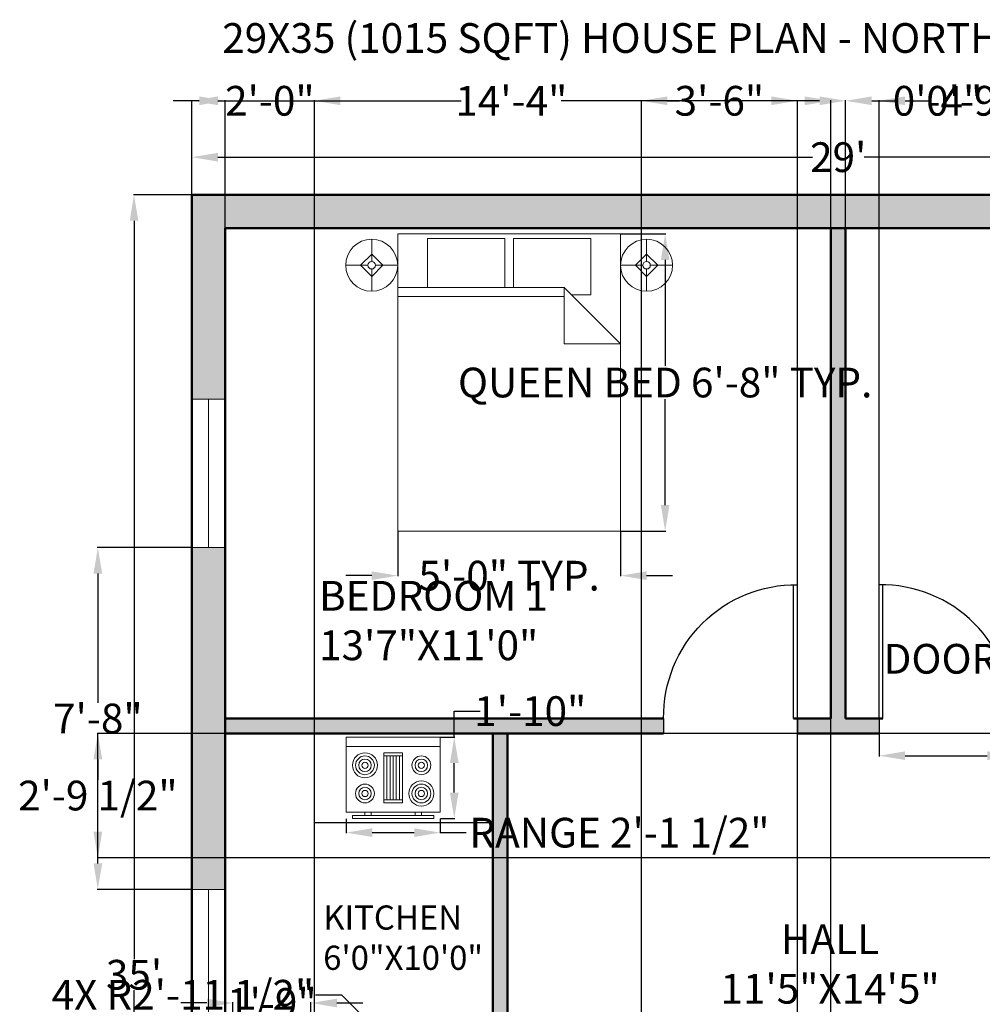
# Model space of a CAD drawing. Units: inches. Extents: x 808573 to 809030, y 884276 to 884799.
# Tile 3 of 4: x 808573 to 808832, y 884534 to 884799. Entities that reach past the tile are written whole.
import ezdxf

# ---------------------------------------------------------------- set-up
doc = ezdxf.new("R2010")
doc.units = ezdxf.units.IN
doc.header["$MEASUREMENT"] = 0
for name, color, linetype, lineweight in [('A-ANNO-DIMS', 2, 'Continuous', 18), ('A-ANNO-TEXT', 7, 'Continuous', 25), ('A-AREA-IDEN', 7, 'Continuous', 25), ('A-DOOR', 3, 'Continuous', 25), ('A-EQPM', 9, 'Continuous', 18), ('A-FLOR-CASE', 9, 'Continuous', 25), ('A-FURN', 8, 'Continuous', 18), ('A-GLAZ', 4, 'Continuous', 18), ('A-WALL', 7, 'Continuous', 50)]:
    doc.layers.add(name, color=color, linetype=linetype, lineweight=lineweight)
doc.layers.add('A-WALL-PATT', color=251, linetype='Continuous', lineweight=13, true_color=0x636466)
doc.styles.get("Standard").update_dxf_attribs({"font": 'arial.ttf'})
doc.dimstyles.get("Standard").update_dxf_attribs({"dimtxt": 8, "dimasz": 7, "dimexe": 0.18, "dimexo": 0.0625, "dimgap": 0.09, "dimtad": 0, "dimtih": 1, "dimtoh": 1, "dimdec": 0, "dimzin": 0, "dimdsep": 46, "dimlunit": 3, "dimtxsty": 'Standard', "dimcen": 0.09, "dimadec": 0, "dimazin": 0, "dimtfac": 1, "dimtdec": 0, "dimtofl": 0, "dimtmove": 0, "dimatfit": 3, "dimfxl": 1, "dimtolj": 1, "dimtzin": 0, "dimarcsym": 0})

# ---------------------------------------------------------------- blocks, each defined once
blk = doc.blocks.new('Range-Oven - 30 in top')
for p, q in [((0, -3), (30, -3)), ((12, -6), (18, -6)), ((13, -20), (13, -6)), ((14, -6), (14, -20)), ((15, -20), (15, -6)), ((16, -6), (16, -20)), ((17, -20), (17, -6)), ((18, -20), (12, -20)), ((6, -24), (6, -25)), ((8, -25), (8, -24)), ((22, -25), (22, -24)), ((24, -24), (24, -25))]:
    blk.add_line(p, q)
for points in [[(0, -24), (0, 0), (30, 0), (30, -24)], [(12, -21), (12, -5), (18, -5), (18, -21)], [(2, -26), (2, -25), (28, -25), (28, -26)]]:
    blk.add_lwpolyline(points, close=True)
for centre, radius in [((6, -9), 4), ((6, -9), 3), ((24, -9), 3), ((6, -9), 2), ((6, -9), 1), ((24, -9), 2), ((24, -9), 1), ((6, -18), 3), ((24, -18), 4), ((24, -18), 3), ((6, -18), 2), ((6, -18), 1), ((24, -18), 2), ((24, -18), 1)]:
    blk.add_circle(centre, radius)
blk = doc.blocks.new('Bed - Queen')
for p, q in [((0, -80.00003), (0, 0)), ((0, 0), (59.99999, 0)), ((59.99999, 0), (59.99999, -80.00003)), ((7.99999, -1.2), (28.79998, -1.2)), ((7.99999, -14.4), (7.99999, -1.2)), ((28.79998, -1.2), (28.79998, -14.4)), ((31.19999, -1.2), (51.99999, -1.2)), ((31.19999, -14.4), (31.19999, -1.2)), ((51.99999, -1.2), (51.99999, -16.4)), ((0, -14.4), (44.8, -14.4)), ((59.99999, -29.6), (44.8, -14.4)), ((44.8, -14.4), (44.8, -29.6)), ((44.8, -16.8), (0, -16.8)), ((51.99999, -16.4), (46.79936, -16.4)), ((44.8, -29.6), (59.99999, -29.6)), ((59.99999, -80.00003), (0, -80.00003))]:
    blk.add_line(p, q)
blk = doc.blocks.new('Lamp - Table')
for p, q in [((0, 7), (0, 1)), ((0, 3), (-3, 0)), ((3, 0), (0, 3)), ((-1, 0), (-7, 0)), ((-3, 0), (0, -3)), ((0, -3), (3, 0)), ((1, 0), (7, 0)), ((0, -1), (0, -7))]:
    blk.add_line(p, q)
for radius in [7, 1]:
    blk.add_circle((0, 0), radius)
blk = doc.blocks.new('*D6')
at = {"layer": 'A-ANNO-DIMS', "color": 0, "lineweight": -2, "transparency": 16777216}
for p, q in [((808619.63, 884751.7), (808619.63, 884761.94)), ((808626.63, 884761.76), (808786.68, 884761.76)), ((808960.63, 884761.76), (808800.58, 884761.76)), ((808967.63, 884751.7), (808967.63, 884761.94))]:
    blk.add_line(p, q, dxfattribs=at)
at = {"layer": 'A-ANNO-DIMS', "color": 0, "transparency": 16777216}
for points in [[(808626.63, 884762.92), (808626.63, 884760.59), (808619.63, 884761.76)], [(808960.63, 884762.92), (808960.63, 884760.59), (808967.63, 884761.76)]]:
    blk.add_solid(points, dxfattribs=at)
at = {"layer": 'Defpoints', "color": 0, "transparency": 16777216}
for p in [(808967.63, 884761.76), (808619.63, 884751.64), (808967.63, 884751.64)]:
    blk.add_point(p, dxfattribs=at)
at = {"layer": 'A-ANNO-DIMS', "color": 0, "transparency": 16777216, "insert": (808793.63, 884761.76), "char_height": 8, "attachment_point": 5}
blk.add_mtext("\\A1;29'", dxfattribs=at)
blk = doc.blocks.new('*D7')
at = {"layer": 'A-ANNO-DIMS', "color": 0, "lineweight": -2, "transparency": 16777216}
for p, q in [((808619.57, 884751.64), (808603.89, 884751.64)), ((808604.07, 884744.64), (808604.07, 884545.82)), ((808604.07, 884338.64), (808604.07, 884537.46)), ((808619.57, 884331.64), (808603.89, 884331.64))]:
    blk.add_line(p, q, dxfattribs=at)
at = {"layer": 'A-ANNO-DIMS', "color": 0, "transparency": 16777216}
for points in [[(808602.9, 884744.64), (808605.23, 884744.64), (808604.07, 884751.64)], [(808602.9, 884338.64), (808605.23, 884338.64), (808604.07, 884331.64)]]:
    blk.add_solid(points, dxfattribs=at)
at = {"layer": 'Defpoints', "color": 0, "transparency": 16777216}
for p in [(808619.63, 884751.64), (808604.07, 884331.64), (808619.63, 884331.64)]:
    blk.add_point(p, dxfattribs=at)
at = {"layer": 'A-ANNO-DIMS', "color": 0, "transparency": 16777216, "insert": (808604.07, 884541.64), "char_height": 8, "attachment_point": 5}
blk.add_mtext("\\A1;35'", dxfattribs=at)
blk = doc.blocks.new('DOOR-SWING-36IN')
for p, q in [((0, 0), (0, 36)), ((1, 0), (1, 36)), ((0, 0), (0, -4)), ((36, 0), (36, -4))]:
    blk.add_line(p, q)
blk.add_arc((0.5, 0.5), 35.5, 359.1931, 90.8069)
blk = doc.blocks.new('WIN-40IN')
for p, q in [((0, 0), (9, 0)), ((4.5, 0), (4.5, -40)), ((0, -40), (9, -40))]:
    blk.add_line(p, q)
blk = doc.blocks.new('WIN-36IN')
for p, q in [((0, 0), (-9, 0)), ((-4.5, 0), (-4.5, -36)), ((0, -36), (-9, -36))]:
    blk.add_line(p, q)
blk = doc.blocks.new('*D17')
at = {"layer": 'A-ANNO-DIMS', "color": 0, "lineweight": -2, "transparency": 16777216}
for p, q in [((808735.1, 884741.09), (808747.22, 884741.09)), ((808747.04, 884734.09), (808747.04, 884705.56)), ((808747.04, 884668.09), (808747.04, 884696.62)), ((808735.1, 884661.09), (808747.22, 884661.09))]:
    blk.add_line(p, q, dxfattribs=at)
at = {"layer": 'A-ANNO-DIMS', "color": 0, "transparency": 16777216}
for points in [[(808745.88, 884734.09), (808748.21, 884734.09), (808747.04, 884741.09)], [(808745.88, 884668.09), (808748.21, 884668.09), (808747.04, 884661.09)]]:
    blk.add_solid(points, dxfattribs=at)
at = {"layer": 'Defpoints', "color": 0, "transparency": 16777216}
for p in [(808735.04, 884741.09), (808747.04, 884741.09), (808735.04, 884661.09)]:
    blk.add_point(p, dxfattribs=at)
at = {"layer": 'A-ANNO-DIMS', "color": 0, "transparency": 16777216, "insert": (808747.04, 884701.09), "char_height": 8, "attachment_point": 5}
blk.add_mtext('\\A1;QUEEN BED 6\'-8" TYP.', dxfattribs=at)
blk = doc.blocks.new('*D18')
at = {"layer": 'A-ANNO-DIMS', "color": 0, "lineweight": -2, "transparency": 16777216}
for p, q in [((808675.04, 884661.03), (808675.04, 884648.91)), ((808735.04, 884661.03), (808735.04, 884648.91)), ((808668.04, 884649.09), (808661.04, 884649.09)), ((808742.04, 884649.09), (808749.04, 884649.09))]:
    blk.add_line(p, q, dxfattribs=at)
at = {"layer": 'A-ANNO-DIMS', "color": 0, "transparency": 16777216}
for points in [[(808668.04, 884650.26), (808668.04, 884647.92), (808675.04, 884649.09)], [(808742.04, 884650.26), (808742.04, 884647.92), (808735.04, 884649.09)]]:
    blk.add_solid(points, dxfattribs=at)
at = {"layer": 'Defpoints', "color": 0, "transparency": 16777216}
for p in [(808675.04, 884661.09), (808735.04, 884661.09), (808735.04, 884649.09)]:
    blk.add_point(p, dxfattribs=at)
at = {"layer": 'A-ANNO-DIMS', "color": 0, "transparency": 16777216, "insert": (808705.04, 884649.09), "char_height": 8, "attachment_point": 5}
blk.add_mtext('\\A1;5\'-0" TYP.', dxfattribs=at)
blk = doc.blocks.new('*D19')
at = {"layer": 'A-ANNO-DIMS', "color": 0, "lineweight": -2, "transparency": 16777216}
for p, q in [((808840.83, 884646.78), (808846.96, 884646.78)), ((808846.78, 884639.78), (808846.78, 884630.94)), ((808846.78, 884613.64), (808846.78, 884622.48)), ((808840.83, 884606.64), (808846.96, 884606.64))]:
    blk.add_line(p, q, dxfattribs=at)
at = {"layer": 'A-ANNO-DIMS', "color": 0, "transparency": 16777216}
for points in [[(808845.62, 884639.78), (808847.95, 884639.78), (808846.78, 884646.78)], [(808845.62, 884613.64), (808847.95, 884613.64), (808846.78, 884606.64)]]:
    blk.add_solid(points, dxfattribs=at)
at = {"layer": 'Defpoints', "color": 0, "transparency": 16777216}
for p in [(808840.76, 884646.78), (808846.78, 884646.78), (808840.76, 884606.64)]:
    blk.add_point(p, dxfattribs=at)
at = {"layer": 'A-ANNO-DIMS', "color": 0, "transparency": 16777216, "insert": (808846.78, 884626.71), "char_height": 8, "attachment_point": 5}
blk.add_mtext('\\A1;DOOR 3\'-4" TYP.', dxfattribs=at)
blk = doc.blocks.new('*D20')
at = {"layer": 'A-ANNO-DIMS', "color": 0, "lineweight": -2, "transparency": 16777216}
for p, q in [((808804.63, 884606.58), (808804.63, 884600.44)), ((808840.76, 884606.58), (808840.76, 884600.44)), ((808811.63, 884600.62), (808833.76, 884600.62)), ((808840.76, 884600.62), (808847.76, 884600.62))]:
    blk.add_line(p, q, dxfattribs=at)
at = {"layer": 'A-ANNO-DIMS', "color": 0, "transparency": 16777216}
for points in [[(808811.63, 884601.79), (808811.63, 884599.45), (808804.63, 884600.62)], [(808833.76, 884601.79), (808833.76, 884599.45), (808840.76, 884600.62)]]:
    blk.add_solid(points, dxfattribs=at)
at = {"layer": 'Defpoints', "color": 0, "transparency": 16777216}
for p in [(808804.63, 884606.64), (808840.76, 884606.64), (808840.76, 884600.62)]:
    blk.add_point(p, dxfattribs=at)
at = {"layer": 'A-ANNO-DIMS', "color": 0, "transparency": 16777216, "insert": (808872.23, 884600.62), "char_height": 8, "attachment_point": 5}
blk.add_mtext('\\A1;3\'-0" TYP.', dxfattribs=at)
blk = doc.blocks.new('*D29')
at = {"layer": 'A-ANNO-DIMS', "color": 0, "lineweight": -2, "transparency": 16777216}
for p, q in [((808661.18, 884583.63), (808661.18, 884579.72)), ((808686.48, 884583.63), (808686.48, 884579.72)), ((808668.18, 884579.9), (808679.48, 884579.9)), ((808686.48, 884579.9), (808693.48, 884579.9))]:
    blk.add_line(p, q, dxfattribs=at)
at = {"layer": 'A-ANNO-DIMS', "color": 0, "transparency": 16777216}
for points in [[(808668.18, 884581.07), (808668.18, 884578.74), (808661.18, 884579.9)], [(808679.48, 884581.07), (808679.48, 884578.74), (808686.48, 884579.9)]]:
    blk.add_solid(points, dxfattribs=at)
at = {"layer": 'Defpoints', "color": 0, "transparency": 16777216}
for p in [(808661.18, 884583.7), (808686.48, 884583.7), (808686.48, 884579.9)]:
    blk.add_point(p, dxfattribs=at)
at = {"layer": 'A-ANNO-DIMS', "color": 0, "transparency": 16777216, "insert": (808734.74, 884579.9), "char_height": 8, "attachment_point": 5}
blk.add_mtext('\\A1;RANGE 2\'-1 1/2"', dxfattribs=at)
blk = doc.blocks.new('*D30')
at = {"layer": 'A-ANNO-DIMS', "color": 0, "lineweight": -2, "transparency": 16777216}
for p, q in [((808690.27, 884605.62), (808690.27, 884612.62)), ((808690.27, 884612.62), (808697.27, 884612.62)), ((808686.54, 884605.62), (808690.45, 884605.62)), ((808690.27, 884590.7), (808690.27, 884598.62)), ((808686.54, 884583.7), (808690.45, 884583.7))]:
    blk.add_line(p, q, dxfattribs=at)
at = {"layer": 'A-ANNO-DIMS', "color": 0, "transparency": 16777216}
for points in [[(808689.1, 884598.62), (808691.44, 884598.62), (808690.27, 884605.62)], [(808689.1, 884590.7), (808691.44, 884590.7), (808690.27, 884583.7)]]:
    blk.add_solid(points, dxfattribs=at)
at = {"layer": 'Defpoints', "color": 0, "transparency": 16777216}
for p in [(808686.48, 884605.62), (808690.27, 884605.62), (808686.48, 884583.7)]:
    blk.add_point(p, dxfattribs=at)
at = {"layer": 'A-ANNO-DIMS', "color": 0, "transparency": 16777216, "insert": (808710.73, 884612.62), "char_height": 8, "attachment_point": 5}
blk.add_mtext('\\A1;1\'-10"', dxfattribs=at)
blk = doc.blocks.new('*D32')
at = {"layer": 'A-ANNO-DIMS', "color": 0, "lineweight": -2, "transparency": 16777216}
for p, q in [((808623.67, 884534.04), (808616.67, 884534.04)), ((808630.67, 884528.7), (808630.67, 884534.22)), ((808651.67, 884528.7), (808651.67, 884534.22)), ((808658.67, 884534.04), (808665.67, 884534.04))]:
    blk.add_line(p, q, dxfattribs=at)
at = {"layer": 'A-ANNO-DIMS', "color": 0, "transparency": 16777216}
for points in [[(808623.67, 884535.2), (808623.67, 884532.87), (808630.67, 884534.04)], [(808658.67, 884535.2), (808658.67, 884532.87), (808651.67, 884534.04)]]:
    blk.add_solid(points, dxfattribs=at)
at = {"layer": 'Defpoints', "color": 0, "transparency": 16777216}
for p in [(808651.67, 884534.04), (808630.67, 884528.64), (808651.67, 884528.64)]:
    blk.add_point(p, dxfattribs=at)
at = {"layer": 'A-ANNO-DIMS', "color": 0, "transparency": 16777216, "insert": (808641.17, 884534.04), "char_height": 8, "attachment_point": 5}
blk.add_mtext('\\A1;1\'-9"', dxfattribs=at)
blk = doc.blocks.new('*D35')
at = {"layer": 'A-ANNO-DIMS', "color": 0, "lineweight": -2, "transparency": 16777216}
for p, q in [((808619.57, 884656.64), (808594.15, 884656.64)), ((808594.33, 884649.64), (808594.33, 884614.81)), ((808594.33, 884571.64), (808594.33, 884606.47)), ((808619.57, 884564.64), (808594.15, 884564.64))]:
    blk.add_line(p, q, dxfattribs=at)
at = {"layer": 'A-ANNO-DIMS', "color": 0, "transparency": 16777216}
for points in [[(808593.16, 884649.64), (808595.5, 884649.64), (808594.33, 884656.64)], [(808593.16, 884571.64), (808595.5, 884571.64), (808594.33, 884564.64)]]:
    blk.add_solid(points, dxfattribs=at)
at = {"layer": 'Defpoints', "color": 0, "transparency": 16777216}
for p in [(808594.33, 884656.64), (808619.63, 884656.64), (808619.63, 884564.64)]:
    blk.add_point(p, dxfattribs=at)
at = {"layer": 'A-ANNO-DIMS', "color": 0, "transparency": 16777216, "insert": (808594.33, 884610.64), "char_height": 8, "attachment_point": 5}
blk.add_mtext('\\A1;7\'-8"', dxfattribs=at)
blk = doc.blocks.new('*D40')
at = {"layer": 'A-ANNO-DIMS', "color": 0, "lineweight": -2, "transparency": 16777216}
for p, q in [((808619.63, 884331.7), (808619.63, 884777.12)), ((808626.63, 884776.94), (808692.17, 884776.94)), ((808784.63, 884776.94), (808719.08, 884776.94)), ((808791.63, 884331.7), (808791.63, 884777.12))]:
    blk.add_line(p, q, dxfattribs=at)
at = {"layer": 'A-ANNO-DIMS', "color": 0, "transparency": 16777216}
for points in [[(808626.63, 884778.11), (808626.63, 884775.77), (808619.63, 884776.94)], [(808784.63, 884778.11), (808784.63, 884775.77), (808791.63, 884776.94)]]:
    blk.add_solid(points, dxfattribs=at)
at = {"layer": 'Defpoints', "color": 0, "transparency": 16777216}
for p in [(808791.63, 884776.94), (808619.63, 884331.64), (808791.63, 884331.64)]:
    blk.add_point(p, dxfattribs=at)
at = {"layer": 'A-ANNO-DIMS', "color": 0, "transparency": 16777216, "insert": (808705.63, 884776.94), "char_height": 8, "attachment_point": 5}
blk.add_mtext('\\A1;14\'-4"', dxfattribs=at)
blk = doc.blocks.new('*D45')
at = {"layer": 'A-ANNO-DIMS', "color": 0, "lineweight": -2, "transparency": 16777216}
for p, q in [((808784.63, 884776.94), (808777.63, 884776.94)), ((808791.63, 884742.7), (808791.63, 884777.12)), ((808795.63, 884742.7), (808795.63, 884777.12)), ((808802.63, 884776.94), (808809.63, 884776.94))]:
    blk.add_line(p, q, dxfattribs=at)
at = {"layer": 'A-ANNO-DIMS', "color": 0, "transparency": 16777216}
for points in [[(808784.63, 884778.11), (808784.63, 884775.77), (808791.63, 884776.94)], [(808802.63, 884778.11), (808802.63, 884775.77), (808795.63, 884776.94)]]:
    blk.add_solid(points, dxfattribs=at)
at = {"layer": 'Defpoints', "color": 0, "transparency": 16777216}
for p in [(808795.63, 884776.94), (808791.63, 884742.64), (808795.63, 884742.64)]:
    blk.add_point(p, dxfattribs=at)
at = {"layer": 'A-ANNO-DIMS', "color": 0, "transparency": 16777216, "insert": (808820.35, 884776.94), "char_height": 8, "attachment_point": 5}
blk.add_mtext('\\A1;0\'-4"', dxfattribs=at)
blk = doc.blocks.new('*D46')
at = {"layer": 'A-ANNO-DIMS', "color": 0, "lineweight": -2, "transparency": 16777216}
for p, q in [((808621.63, 884776.94), (808614.63, 884776.94)), ((808628.63, 884606.7), (808628.63, 884777.12)), ((808652.63, 884582.7), (808652.63, 884777.12)), ((808659.63, 884776.94), (808666.63, 884776.94))]:
    blk.add_line(p, q, dxfattribs=at)
at = {"layer": 'A-ANNO-DIMS', "color": 0, "transparency": 16777216}
for points in [[(808621.63, 884778.11), (808621.63, 884775.77), (808628.63, 884776.94)], [(808659.63, 884778.11), (808659.63, 884775.77), (808652.63, 884776.94)]]:
    blk.add_solid(points, dxfattribs=at)
at = {"layer": 'Defpoints', "color": 0, "transparency": 16777216}
for p in [(808652.63, 884776.94), (808628.63, 884606.64), (808652.63, 884582.64)]:
    blk.add_point(p, dxfattribs=at)
at = {"layer": 'A-ANNO-DIMS', "color": 0, "transparency": 16777216, "insert": (808640.63, 884776.94), "char_height": 8, "attachment_point": 5}
blk.add_mtext('\\A1;2\'-0"', dxfattribs=at)
blk = doc.blocks.new('*D48')
at = {"layer": 'A-ANNO-DIMS', "color": 0, "lineweight": -2, "transparency": 16777216}
for p, q in [((808740.63, 884434.7), (808740.63, 884777.12)), ((808747.63, 884776.94), (808750.91, 884776.94)), ((808775.63, 884776.94), (808772.35, 884776.94)), ((808782.63, 884434.7), (808782.63, 884777.12))]:
    blk.add_line(p, q, dxfattribs=at)
at = {"layer": 'A-ANNO-DIMS', "color": 0, "transparency": 16777216}
for points in [[(808747.63, 884778.11), (808747.63, 884775.77), (808740.63, 884776.94)], [(808775.63, 884778.11), (808775.63, 884775.77), (808782.63, 884776.94)]]:
    blk.add_solid(points, dxfattribs=at)
at = {"layer": 'Defpoints', "color": 0, "transparency": 16777216}
for p in [(808782.63, 884776.94), (808740.63, 884434.64), (808782.63, 884434.64)]:
    blk.add_point(p, dxfattribs=at)
at = {"layer": 'A-ANNO-DIMS', "color": 0, "transparency": 16777216, "insert": (808761.63, 884776.94), "char_height": 8, "attachment_point": 5}
blk.add_mtext('\\A1;3\'-6"', dxfattribs=at)
blk = doc.blocks.new('*D49')
at = {"layer": 'A-ANNO-DIMS', "color": 0, "lineweight": -2, "transparency": 16777216}
for p, q in [((808788.63, 884776.94), (808781.63, 884776.94)), ((808795.63, 884610.7), (808795.63, 884777.12)), ((808804.63, 884610.7), (808804.63, 884777.12)), ((808811.63, 884776.94), (808818.63, 884776.94))]:
    blk.add_line(p, q, dxfattribs=at)
at = {"layer": 'A-ANNO-DIMS', "color": 0, "transparency": 16777216}
for points in [[(808788.63, 884778.11), (808788.63, 884775.77), (808795.63, 884776.94)], [(808811.63, 884778.11), (808811.63, 884775.77), (808804.63, 884776.94)]]:
    blk.add_solid(points, dxfattribs=at)
at = {"layer": 'Defpoints', "color": 0, "transparency": 16777216}
for p in [(808804.63, 884776.94), (808795.63, 884610.64), (808804.63, 884610.64)]:
    blk.add_point(p, dxfattribs=at)
at = {"layer": 'A-ANNO-DIMS', "color": 0, "transparency": 16777216, "insert": (808829.35, 884776.94), "char_height": 8, "attachment_point": 5}
blk.add_mtext('\\A1;0\'-9"', dxfattribs=at)
blk = doc.blocks.new('*D52')
at = {"layer": 'A-ANNO-DIMS', "color": 0, "lineweight": -2, "transparency": 16777216}
for p, q in [((808842.57, 884606.64), (808594.15, 884606.64)), ((808594.33, 884599.64), (808594.33, 884594.12)), ((808594.33, 884580.14), (808594.33, 884585.66)), ((808842.57, 884573.14), (808594.15, 884573.14))]:
    blk.add_line(p, q, dxfattribs=at)
at = {"layer": 'A-ANNO-DIMS', "color": 0, "transparency": 16777216}
for points in [[(808593.16, 884599.64), (808595.5, 884599.64), (808594.33, 884606.64)], [(808593.16, 884580.14), (808595.5, 884580.14), (808594.33, 884573.14)]]:
    blk.add_solid(points, dxfattribs=at)
at = {"layer": 'Defpoints', "color": 0, "transparency": 16777216}
for p in [(808842.63, 884606.64), (808594.33, 884573.14), (808842.63, 884573.14)]:
    blk.add_point(p, dxfattribs=at)
at = {"layer": 'A-ANNO-DIMS', "color": 0, "transparency": 16777216, "insert": (808594.33, 884589.89), "char_height": 8, "attachment_point": 5}
blk.add_mtext('\\A1;2\'-9 1/2"', dxfattribs=at)
blk = doc.blocks.new('*D56')
at = {"layer": 'A-ANNO-DIMS', "color": 0, "lineweight": -2, "transparency": 16777216}
for p, q in [((808652.96, 884536.26), (808659.96, 884536.26)), ((808659.96, 884536.26), (808670.07, 884526.14)), ((808700.04, 884496.09), (808700.22, 884496.09)), ((808700.13, 884496), (808700.13, 884496.18))]:
    blk.add_line(p, q, dxfattribs=at)
at = {"layer": 'A-ANNO-DIMS', "color": 0, "transparency": 16777216}
blk.add_solid([(808670.9, 884526.97), (808669.25, 884525.32), (808675.02, 884521.19)], dxfattribs=at)
at = {"layer": 'Defpoints', "color": 0, "transparency": 16777216}
for p in [(808675.02, 884521.19), (808700.13, 884496.09)]:
    blk.add_point(p, dxfattribs=at)
at = {"layer": 'A-ANNO-DIMS', "color": 0, "transparency": 16777216, "insert": (808617.23, 884536.26), "char_height": 8, "attachment_point": 5}
blk.add_mtext('\\A1;4X R2\'-11 1/2"', dxfattribs=at)

msp = doc.modelspace()

# ---------------------------------------------------------------- hatches: boundary and pattern name
at = {"layer": 'A-WALL-PATT'}
h = msp.add_hatch(color=256, dxfattribs=at)
h.dxf.hatch_style = 1
h.paths.add_polyline_path([(808967.63, 884751.64), (808619.63, 884751.64), (808619.63, 884696.64), (808628.63, 884696.64), (808628.63, 884742.64), (808791.63, 884742.64), (808958.63, 884742.64), (808958.63, 884696.64), (808967.63, 884696.64)])
h.paths.add_polyline_path([(808967.63, 884656.64), (808958.63, 884656.64), (808958.63, 884610.64), (808958.63, 884590.14), (808967.63, 884590.14)])
h.paths.add_polyline_path([(808967.63, 884494.64), (808958.63, 884494.64), (808958.63, 884479.64), (808958.63, 884340.64), (808901.23, 884340.64), (808901.23, 884331.64), (808967.63, 884331.64)])
h.paths.add_polyline_path([(808967.63, 884554.14), (808958.63, 884554.14), (808958.63, 884537.64), (808875.63, 884537.64), (808875.63, 884533.64), (808884.63, 884533.64), (808884.63, 884479.64), (808841.63, 884479.64), (808841.63, 884533.64), (808845.63, 884533.64), (808845.63, 884537.64), (808837.63, 884537.64), (808837.63, 884479.64), (808837.63, 884475.64), (808958.63, 884475.64), (808958.63, 884479.64), (808888.63, 884479.64), (808888.63, 884533.64), (808958.63, 884533.64), (808958.63, 884518.64), (808967.63, 884518.64)])
h.paths.add_polyline_path([(808858.03, 884340.64), (808800.63, 884340.64), (808800.63, 884365.64), (808791.63, 884365.64), (808791.63, 884331.64), (808858.03, 884331.64)])
h.paths.add_polyline_path([(808800.63, 884475.64), (808801.63, 884475.64), (808801.63, 884479.64), (808791.63, 884479.64), (808791.63, 884430.64), (808791.63, 884405.64), (808800.63, 884405.64)])
h.paths.add_polyline_path([(808740.63, 884434.64), (808704.63, 884434.64), (808704.63, 884438.64), (808700.63, 884438.64), (808700.63, 884434.64), (808628.63, 884434.64), (808628.63, 884443.64), (808619.63, 884443.64), (808619.63, 884430.64), (808740.63, 884430.64)])
h.paths.add_polyline_path([(808628.63, 884528.64), (808619.63, 884528.64), (808619.63, 884473.64), (808628.63, 884473.64), (808628.63, 884482.64)])
h.paths.add_polyline_path([(808628.63, 884606.64), (808628.63, 884656.64), (808619.63, 884656.64), (808619.63, 884564.64), (808628.63, 884564.64)])
h.paths.add_polyline_path([(808704.63, 884482.64), (808704.63, 884495.59), (808700.63, 884495.59), (808700.63, 884486.64), (808628.63, 884486.64), (808628.63, 884482.64), (808700.63, 884482.64), (808700.63, 884468.64), (808704.63, 884468.64)])
h.paths.add_polyline_path([(808704.63, 884606.64), (808700.63, 884606.64), (808700.63, 884531.59), (808704.63, 884531.59)])
h.paths.add_polyline_path([(808746.63, 884610.64), (808628.63, 884610.64), (808628.63, 884606.64), (808746.63, 884606.64)])
h.paths.add_polyline_path([(808804.63, 884610.64), (808795.63, 884610.64), (808795.63, 884742.64), (808791.63, 884742.64), (808791.63, 884610.64), (808782.63, 884610.64), (808782.63, 884606.64), (808804.63, 884606.64)])
h.paths.add_polyline_path([(808958.63, 884610.64), (808840.63, 884610.64), (808840.63, 884606.64), (808958.63, 884606.64)])

# ---------------------------------------------------------------- linework, layer by layer
at = {"layer": 'A-FLOR-CASE'}
for p, q in [((808652.63, 884486.64), (808652.63, 884582.64)), ((808652.63, 884582.64), (808700.63, 884582.64))]:
    msp.add_line(p, q, dxfattribs=at)
at = {"layer": 'A-WALL'}
for p, q in [((808619.63, 884751.64), (808967.63, 884751.64)), ((808619.63, 884331.64), (808619.63, 884751.64)), ((808628.63, 884742.64), (808791.63, 884742.64)), ((808628.63, 884606.64), (808628.63, 884742.64)), ((808791.63, 884742.64), (808958.63, 884742.64)), ((808791.63, 884610.64), (808791.63, 884742.64)), ((808795.63, 884742.64), (808795.63, 884610.64)), ((808628.63, 884610.64), (808746.63, 884610.64)), ((808781.63, 884610.64), (808791.63, 884610.64)), ((808795.63, 884610.64), (808805.63, 884610.64)), ((808795.63, 884610.64), (808795.63, 884610.64)), ((808795.63, 884610.64), (808804.63, 884610.64)), ((808628.63, 884606.64), (808746.63, 884606.64)), ((808628.63, 884482.64), (808628.63, 884606.64)), ((808700.63, 884531.59), (808700.63, 884606.64)), ((808704.63, 884606.64), (808746.63, 884606.64)), ((808704.63, 884531.59), (808704.63, 884606.64)), ((808782.63, 884606.64), (808804.63, 884606.64)), ((808782.63, 884606.64), (808791.63, 884606.64))]:
    msp.add_line(p, q, dxfattribs=at)

# ---------------------------------------------------------------- block references
at = {"layer": 'A-DOOR', "extrusion": (0, 0, -1), "zscale": -1}
msp.add_blockref('DOOR-SWING-36IN', (-808782.63, 884610.64), dxfattribs=at)
at = {"layer": 'A-DOOR'}
msp.add_blockref('DOOR-SWING-36IN', (808804.63, 884610.64), dxfattribs=at)
at = {"layer": 'A-EQPM', "xscale": 0.8430906105448694, "yscale": 0.8430906105448694, "zscale": 0.8430906105448694}
msp.add_blockref('Range-Oven - 30 in top', (808661.18, 884605.62), dxfattribs=at)
at = {"layer": 'A-FURN'}
for name, p in [('Lamp - Table', (808668.04, 884732.66)), ('Bed - Queen', (808675.04, 884741.09))]:
    msp.add_blockref(name, p, dxfattribs=at)
at = {"layer": 'A-FURN', "xscale": -1}
msp.add_blockref('Lamp - Table', (808742.04, 884732.66), dxfattribs=at)
at = {"layer": 'A-GLAZ', "rotation": 180}
msp.add_blockref('WIN-40IN', (808628.63, 884656.64), dxfattribs=at)
at = {"layer": 'A-GLAZ'}
msp.add_blockref('WIN-36IN', (808628.63, 884564.64), dxfattribs=at)

# ---------------------------------------------------------------- texts
at = {"layer": 'A-ANNO-TEXT', "insert": (808627.8, 884797.84), "char_height": 8, "attachment_point": 1}
msp.add_mtext_dynamic_manual_height_columns('{\\fArial|b1|i0|c0|p34;29X35 (1015 SQFT) HOUSE PLAN - NORTH FACE -FP075}', width=304.7381, gutter_width=1, heights=[0.175], dxfattribs=at)
at = {"layer": 'A-AREA-IDEN', "attachment_point": 1}
for s, insert, char_height in [('BEDROOM 1\\P13\'7"X11\'0"', (808653.87, 884647.67), 8), ('KITCHEN\\P6\'0"X10\'0"', (808654.99, 884560.3), 6.5), ('\\pxqc;HALL\\P11\'5"X14\'5"', (808744.37, 884555.21), 8)]:
    msp.add_mtext_dynamic_manual_height_columns(s, width=94.1107, gutter_width=1, heights=[0], dxfattribs=dict(at, insert=insert, char_height=char_height))

# ---------------------------------------------------------------- dimensions: what is measured, and where the dimension line sits
at = {"layer": 'A-ANNO-DIMS'}
for base, p1, p2, override, picture, middle in [((808652.63, 884776.94), (808628.63, 884606.64), (808652.63, 884582.64), {"dimdec": 1, "dimlfac": 1, "dimrnd": 0, "dimzin": 1, "dimdsep": 46, "dimlunit": 4, "dimfrac": 2}, '*D46', (808640.63, 884776.94)), ((808791.63, 884776.94), (808619.63, 884331.64), (808791.63, 884331.64), {"dimdec": 1, "dimlfac": 1, "dimrnd": 0, "dimzin": 1, "dimdsep": 46, "dimlunit": 4, "dimfrac": 2}, '*D40', (808705.63, 884776.94)), ((808782.63, 884776.94), (808740.63, 884434.64), (808782.63, 884434.64), {"dimdec": 1, "dimlfac": 1, "dimrnd": 0, "dimzin": 1, "dimdsep": 46, "dimlunit": 4, "dimfrac": 2}, '*D48', (808761.63, 884776.94)), ((808795.63, 884776.94), (808791.63, 884742.64), (808795.63, 884742.64), {"dimdec": 1, "dimlfac": 1, "dimrnd": 0, "dimzin": 1, "dimdsep": 46, "dimlunit": 4, "dimfrac": 2}, '*D45', (808820.35, 884776.94)), ((808804.63, 884776.94), (808795.63, 884610.64), (808804.63, 884610.64), {"dimdec": 1, "dimlfac": 1, "dimrnd": 0, "dimzin": 1, "dimdsep": 46, "dimlunit": 4, "dimfrac": 2}, '*D49', (808829.35, 884776.94)), ((808967.63, 884761.76), (808619.63, 884751.64), (808967.63, 884751.64), {"dimclrd": 0, "dimclre": 0, "dimclrt": 0}, '*D6', (808793.63, 884761.76)), ((808651.67, 884534.04), (808630.67, 884528.64), (808651.67, 884528.64), {"dimdec": 1, "dimlfac": 1, "dimrnd": 0, "dimzin": 1, "dimdsep": 46, "dimlunit": 4, "dimfrac": 2}, '*D32', (808641.17, 884534.04))]:
    dim = msp.add_linear_dim(base=base, p1=p1, p2=p2, dimstyle='Standard', override=override, dxfattribs=at)
    dim.commit()
    dim.dimension.update_dxf_attribs({"geometry": picture, "text_midpoint": middle})
for base, p1, p2, override, picture, middle in [((808604.07, 884331.64), (808619.63, 884751.64), (808619.63, 884331.64), {"dimclrd": 0, "dimclre": 0, "dimclrt": 0}, '*D7', (808604.07, 884541.64)), ((808594.33, 884656.64), (808619.63, 884564.64), (808619.63, 884656.64), {"dimdec": 1, "dimlfac": 1, "dimrnd": 0, "dimzin": 1, "dimdsep": 46, "dimlunit": 4, "dimfrac": 2}, '*D35', (808594.33, 884610.64)), ((808690.27, 884605.62), (808686.48, 884583.7), (808686.48, 884605.62), {"dimdec": 1, "dimlfac": 1, "dimrnd": 0, "dimzin": 1, "dimdsep": 46, "dimlunit": 4, "dimfrac": 2}, '*D30', (808710.73, 884612.62)), ((808594.33, 884573.14), (808842.63, 884606.64), (808842.63, 884573.14), {"dimdec": 1, "dimlfac": 1, "dimrnd": 0, "dimzin": 1, "dimdsep": 46, "dimlunit": 4, "dimfrac": 2}, '*D52', (808594.33, 884589.89))]:
    dim = msp.add_linear_dim(base=base, p1=p1, p2=p2, angle=90, dimstyle='Standard', override=override, dxfattribs=at)
    dim.commit()
    dim.dimension.update_dxf_attribs({"geometry": picture, "text_midpoint": middle})
for base, p1, p2, text, picture, middle in [((808747.04, 884741.09), (808735.04, 884661.09), (808735.04, 884741.09), 'QUEEN BED <> TYP.', '*D17', (808747.04, 884701.09)), ((808846.78, 884646.78), (808840.76, 884606.64), (808840.76, 884646.78), 'DOOR <> TYP.', '*D19', (808846.78, 884626.71))]:
    dim = msp.add_linear_dim(base=base, p1=p1, p2=p2, angle=90, text=text, dimstyle='Standard', override={"dimdec": 1, "dimlfac": 1, "dimrnd": 0, "dimzin": 1, "dimdsep": 46, "dimlunit": 4, "dimfrac": 2}, dxfattribs=at)
    dim.commit()
    dim.dimension.update_dxf_attribs({"geometry": picture, "text_midpoint": middle})
for base, p1, p2, text, picture, middle in [((808735.04, 884649.09), (808675.04, 884661.09), (808735.04, 884661.09), '<> TYP.', '*D18', (808705.04, 884649.09)), ((808840.76, 884600.62), (808804.63, 884606.64), (808840.76, 884606.64), '<> TYP.', '*D20', (808872.23, 884600.62)), ((808686.48, 884579.9), (808661.18, 884583.7), (808686.48, 884583.7), 'RANGE <>', '*D29', (808734.74, 884579.9))]:
    dim = msp.add_linear_dim(base=base, p1=p1, p2=p2, text=text, dimstyle='Standard', override={"dimdec": 1, "dimlfac": 1, "dimrnd": 0, "dimzin": 1, "dimdsep": 46, "dimlunit": 4, "dimfrac": 2}, dxfattribs=at)
    dim.commit()
    dim.dimension.update_dxf_attribs({"geometry": picture, "text_midpoint": middle})
dim = msp.add_radius_dim(center=(808700.13, 884496.09), mpoint=(808675.02, 884521.19), text='4X <>', dimstyle='Standard', override={"dimdec": 1, "dimlfac": 1, "dimrnd": 0, "dimzin": 1, "dimdsep": 46, "dimlunit": 4, "dimfrac": 2}, dxfattribs=at)
dim.commit()
dim.dimension.update_dxf_attribs({"geometry": '*D56', "text_midpoint": (808617.23, 884536.26), "dimtype": 164})

doc.saveas('drawing.dxf')
